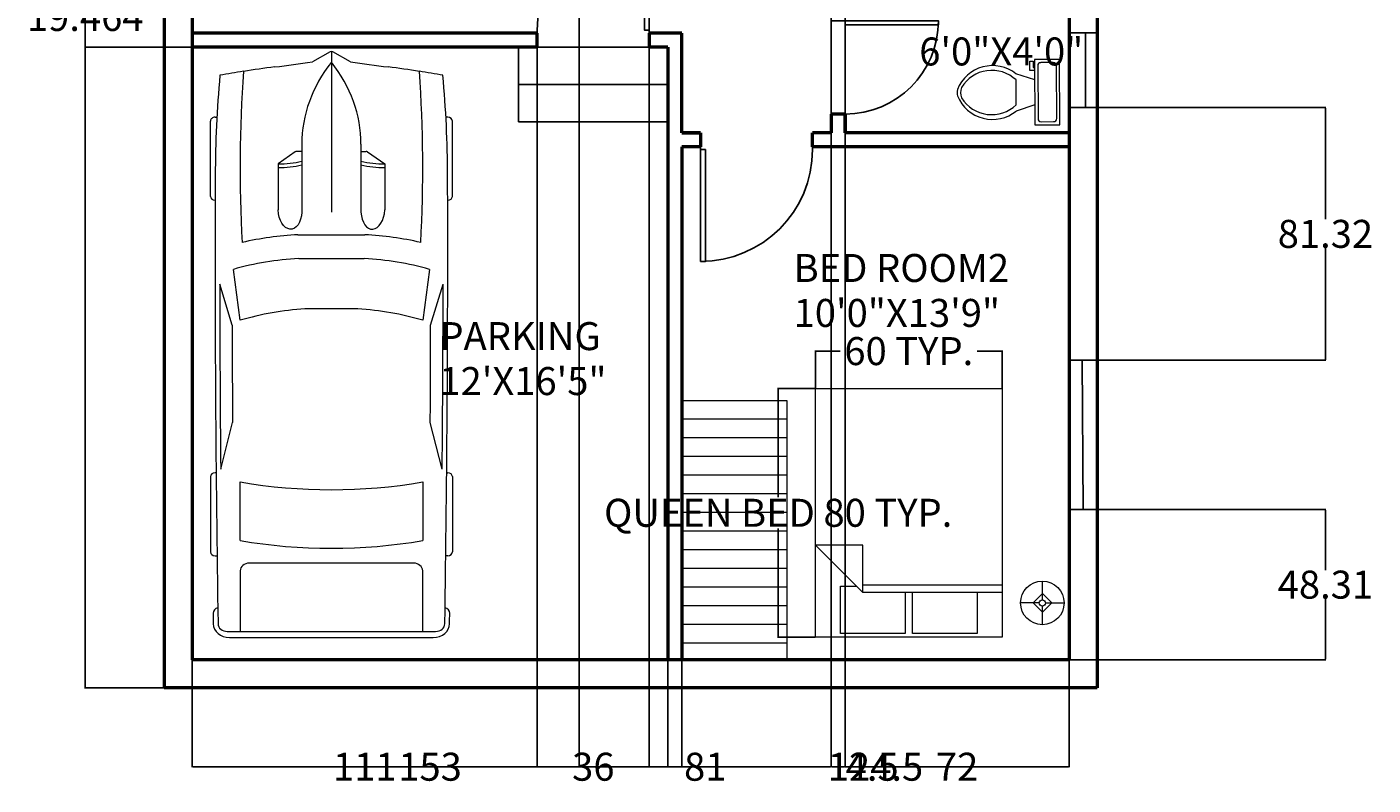
# Model space of a CAD drawing. Units: inches. Extents: x -49 to 419, y 83 to 650.
# Tile 1 of 2: x -14 to 419, y 83 to 327. Entities that reach past the tile are written whole.
import ezdxf

# ---------------------------------------------------------------- set-up
doc = ezdxf.new("R2010")
doc.units = ezdxf.units.IN
for name, color, linetype, lineweight in [('A-ANNO-DIMS', 2, 'Continuous', 18), ('A-AREA-IDEN', 2, 'Continuous', 25), ('A-DOOR', 20, 'Continuous', 25), ('A-FLOR-CASE', 130, 'Continuous', 18), ('A-FLOR-FIXT', 130, 'Continuous', 18), ('A-FLOR-STRS', 150, 'Continuous', 25), ('A-GLAZ', 70, 'Continuous', 25), ('A-SITE-VEHI', 130, 'Continuous', 13), ('FUR', 130, 'Continuous', 18), ('WAL', 210, 'Continuous', 50)]:
    doc.layers.add(name, color=color, linetype=linetype, lineweight=lineweight)
doc.styles.get("Standard").update_dxf_attribs({"font": 'arial.ttf', "height": 9})
doc.dimstyles.get("Standard").update_dxf_attribs({"dimtxt": 0.18, "dimasz": 0.18, "dimexe": 0.18, "dimexo": 0.0625, "dimgap": 0.09, "dimtad": 0, "dimtih": 1, "dimtoh": 1, "dimdec": 4, "dimzin": 0, "dimdsep": 46, "dimtxsty": 'Standard', "dimcen": 0.09, "dimadec": 0, "dimazin": 0, "dimtfac": 1, "dimtdec": 4, "dimtofl": 0, "dimtmove": 0, "dimatfit": 3, "dimfxl": 1, "dimtolj": 1, "dimtzin": 0, "dimarcsym": 0})

# ---------------------------------------------------------------- blocks, each defined once
blk = doc.blocks.new('*U2')
for p, q in [((0, 0), (0, -6)), ((40, 0), (40, -6))]:
    blk.add_line(p, q)
blk.add_lwpolyline([(0, 0), (0, 40), (1.75, 40), (1.75, 0)], close=True)
blk.add_arc((0, 0), 40, 0, 90)
blk = doc.blocks.new('*U4')
for p, q in [((9.5, -6), (9.5, -2)), ((-10, -8.5), (-8, -8.5)), ((-10, -9.5), (-10, -8.5)), ((-8, -8.5), (-8, -8)), ((-7, -8), (-7, -9.5)), ((-4, -8), (-6, -14)), ((4, -8), (6, -14)), ((-7, -9.5), (-10, -9.5)), ((4, -14), (-4, -14))]:
    blk.add_line(p, q)
blk.add_lwpolyline([(10.5, -8), (10.5, 0), (-10.5, 0), (-10.5, -8)], close=True)
for points in [[(-9.5, -2), (-9.5, -6)], [(8.5, -1), (-8.5, -1)], [(-8.5, -7), (8.5, -7)]]:
    blk.add_lwpolyline(points)
for centre, radius, start, end in [((-8.62, -1.88), 0.884, 81.8699, 188.1301), ((8.62, -1.88), 0.884, 351.8699, 98.1301), ((-8.62, -6.12), 0.884, 171.8699, 278.1301), ((8.62, -6.12), 0.884, 261.8699, 8.1301), ((3.52, -21.58), 12.17, 141.4691, 247.9714), ((4.2, -21.82), 11.33, 136.3677, 238.9468), ((-3.52, -21.58), 12.17, 292.0284, 38.5307), ((-4.2, -21.82), 11.33, 301.053, 43.6321), ((0, -27.88), 4, 245.7318, 294.2682), ((0, -29), 4, 254.8605, 285.1395)]:
    blk.add_arc(centre, radius, start, end)
blk = doc.blocks.new('Bed - Queen')
for p, q in [((0, -80.00003), (0, 0)), ((0, 0), (59.99999, 0)), ((59.99999, 0), (59.99999, -80.00003)), ((7.99999, -1.2), (28.79998, -1.2)), ((7.99999, -14.4), (7.99999, -1.2)), ((28.79998, -1.2), (28.79998, -14.4)), ((31.19999, -1.2), (51.99999, -1.2)), ((31.19999, -14.4), (31.19999, -1.2)), ((51.99999, -1.2), (51.99999, -16.4)), ((0, -14.4), (44.8, -14.4)), ((44.8, -16.8), (0, -16.8)), ((59.99999, -29.6), (44.8, -14.4)), ((44.8, -14.4), (44.8, -29.6)), ((51.99999, -16.4), (46.79936, -16.4)), ((44.8, -29.6), (59.99999, -29.6)), ((59.99999, -80.00003), (0, -80.00003))]:
    blk.add_line(p, q)
blk = doc.blocks.new('Lamp - Table')
for p, q in [((0, 7), (0, 1)), ((-1, 0), (-7, 0)), ((0, 3), (-3, 0)), ((-3, 0), (0, -3)), ((3, 0), (0, 3)), ((0, -3), (3, 0)), ((1, 0), (7, 0)), ((0, -1), (0, -7))]:
    blk.add_line(p, q)
for radius in [7, 1]:
    blk.add_circle((0, 0), radius)
blk = doc.blocks.new('*U11')
for p, q in [((21.1, 37.41), (21.1, 36.83)), ((46.55, 38.89), (22.35, 38.89)), ((47.8, 37.39), (47.8, 37.41)), ((87.99, 31.87), (74.76, 35.92)), ((134.31, 35.6), (119.29, 31.78)), ((135.45, 37.07), (135.45, 37.41)), ((136.7, 38.89), (160.9, 38.89)), ((162.15, 37.41), (162.15, 36.77)), ((70.03, 31.54), (86.41, 29.35)), ((186.47, -33.5), (186.47, 33.5)), ((188.4, -32.76), (188.4, 32.76)), ((138.42, 29.35), (157.25, 29.35)), ((164.52, 26.39), (164.52, -26.39)), ((186.47, 29.35), (167.01, 29.35)), ((32.27, 11.63), (36.13, 17.17)), ((36.13, 17.17), (50.94, 17.17)), ((29.77, 9.51), (51.68, 9.51)), ((32.12, 9.51), (32.12, 11.15)), ((58.92, -10.77), (58.92, 10.77)), ((66.55, -10.53), (66.55, 10.53)), ((186.47, -10.53), (186.47, 10.53)), ((3.27, 6.13), (0.1, 0.41)), ((82.74, 8.5), (82.74, -8.5)), ((0, 0), (51.68, 0)), ((0.1, -0.41), (3.27, -6.13)), ((29.77, -9.51), (51.68, -9.51)), ((32.12, -9.51), (32.12, -11.15)), ((32.27, -11.63), (36.13, -17.17)), ((36.13, -17.17), (50.94, -17.17)), ((86.41, -29.35), (70.03, -31.54)), ((157.25, -29.35), (138.42, -29.35)), ((167.01, -29.35), (186.47, -29.35)), ((87.99, -31.87), (74.76, -35.92)), ((134.31, -35.6), (119.29, -31.78)), ((21.1, -37.41), (21.1, -36.83)), ((46.55, -38.89), (22.35, -38.89)), ((47.8, -37.39), (47.8, -37.41)), ((135.45, -37.07), (135.45, -37.41)), ((136.7, -38.89), (160.9, -38.89)), ((162.15, -37.41), (162.15, -36.77))]:
    blk.add_line(p, q)
for centre, major_axis, ratio, start_param, end_param in [((266.03, -27.52), (0, 313.31), 0.842304, 1.367076, 1.39176), ((41.19, -490.86), (0, 528.23), 0.842304, 0.00281, 0.075598), ((22.35, 37.41), (0, -1.48), 0.842304, 3.141593, 4.712389), ((64.48, -10555.62), (0, 10593.03), 0.842304, -0.013397, 0.002797), ((46.55, 37.41), (0, 1.48), 0.842304, -1.570796, 0), ((64.48, -10555.62), (0, -10591.55), 0.842304, 3.133765, 3.140441), ((136.7, 37.41), (0, -1.48), 0.842304, 3.141593, 4.712389), ((160.9, 37.41), (0, 1.48), 0.842304, -1.570796, 0), ((180.63, 35.84), (0, 2.22), 0.842304, -0.013017, 1.249894), ((64.48, -10556.36), (0, 10595.31), 0.842304, -0.013397, -0.013017), ((183.98, 33.5), (0, -2.96), 0.842304, 1.570796, 3.128196), ((183.98, 32.76), (0, -5.25), 0.842304, 1.570796, 3.128196), ((135.29, 5.39), (0, 81.77), 0.842304, 1.245306, 1.50788), ((95.79, -3666.35), (0, -3698.24), 0.842304, 3.134049, 3.144098), ((259.18, -27.52), (0, -305.3), 0.842304, 4.528606, 4.561838), ((37.47, -593.96), (0, -623.33), 0.842304, 3.096046, 3.200911), ((134.4, 5.39), (0, -89.78), 0.842304, 4.449482, 4.652344), ((149.6, 2.8), (0, -79.58), 0.842304, 4.372215, 4.640744), ((17.08, 0), (0, 147.02), 0.842304, 4.511394, 4.913384), ((35.91, 0), (0, 147.02), 0.842304, 4.511394, 4.913384), ((167.01, 26.39), (0, 2.96), 0.842304, 0, 1.570796), ((-204.49, 52.4), (0, -250.96), 0.842304, 1.385369, 1.434372), ((13.04, 17.01), (0, 27.42), 0.842304, 4.435146, 4.718221), ((14.2, 17.01), (0, 27.42), 0.842304, 4.435146, 4.718221), ((50.79, 13.34), (6.34, -0.36), 0.603834, -1.395552, 1.581315), ((29.77, -46.66), (0, 56.17), 0.842304, 0, 0.590319), ((32.75, 11.15), (0, 0.74), 0.842304, 0.879714, 1.570796), ((0.62, 0), (0, -0.74), 0.842304, 4.131459, 5.293319), ((29.77, 46.66), (0, 56.17), 0.842304, 2.551274, 3.141593), ((-204.49, -52.4), (0, 250.96), 0.842304, -1.434372, -1.385369), ((149.6, -2.8), (0, -79.58), 0.842304, -1.499151, -1.230623), ((32.75, -11.15), (0, -0.74), 0.842304, 4.712389, 5.403472), ((13.04, -17.01), (0, -27.42), 0.842304, 1.564964, 1.848039), ((14.2, -17.01), (0, -27.42), 0.842304, 1.564964, 1.848039), ((134.4, -5.39), (0, -89.78), 0.842304, -1.510751, -1.307889), ((135.29, -5.39), (0, -81.77), 0.842304, -1.50788, -1.245306), ((259.18, 27.52), (0, 305.3), 0.842304, 1.721348, 1.754579), ((266.03, 27.52), (0, 313.31), 0.842304, 1.749832, 1.774517), ((37.47, 593.96), (0, -623.33), 0.842304, -0.059319, 0.045547), ((167.01, -26.39), (0, -2.96), 0.842304, 4.712389, 6.283185), ((95.79, 3666.35), (0, -3698.24), 0.842304, -0.002505, 0.007544), ((183.98, -33.5), (0, 2.96), 0.842304, 3.15499, 4.712389), ((183.98, -32.76), (0, -5.25), 0.842304, 0.013397, 1.570796), ((41.19, 490.86), (0, -528.23), 0.842304, -0.075598, -0.00281), ((22.35, -37.41), (0, 1.48), 0.842304, 1.570796, 3.141593), ((64.48, 10555.62), (0, 10593.03), 0.842304, 3.138796, 3.15499), ((46.55, -37.41), (0, -1.48), 0.842304, 0, 1.570796), ((64.48, 10555.62), (0, -10591.55), 0.842304, 0.001152, 0.007828), ((136.7, -37.41), (0, -1.48), 0.842304, -1.570796, 0), ((160.9, -37.41), (0, 1.48), 0.842304, 3.141593, 4.712389), ((180.63, -35.84), (0, -2.22), 0.842304, -1.249894, 0.013017), ((64.48, 10556.36), (0, 10595.31), 0.842304, 3.15461, 3.15499)]:
    blk.add_ellipse(centre, major_axis=major_axis, ratio=ratio, start_param=start_param, end_param=end_param)
at = {"extrusion": (0, 0, -1)}
blk.add_ellipse((50.79, -13.34), major_axis=(6.34, 0.36), ratio=0.603834, start_param=-1.395552, end_param=1.581315, dxfattribs=at)
blk = doc.blocks.new('WIN-48IN')
for p, q in [((0, 48), (0, 0)), ((9, 48), (0, 48)), ((4.19, 48), (4.5, 0)), ((9, 0), (9, 48)), ((0, 0), (9, 0))]:
    blk.add_line(p, q)
blk = doc.blocks.new('WIN-24IN')
for p, q in [((0, 24), (0, 0)), ((9, 24), (0, 24)), ((0, 24), (5.33, 24)), ((5.33, 24), (5.33, 0)), ((9, 0), (9, 24)), ((0, 0), (9, 0))]:
    blk.add_line(p, q)
blk = doc.blocks.new('*D18')
at = {"layer": 'A-ANNO-DIMS', "color": 0, "lineweight": -2, "transparency": 16777216}
for p, q in [((239.4, 210.27), (227.28, 210.27)), ((227.46, 210.09), (227.46, 175.29)), ((227.46, 130.45), (227.46, 165.25)), ((239.4, 130.27), (227.28, 130.27))]:
    blk.add_line(p, q, dxfattribs=at)
at = {"layer": 'A-ANNO-DIMS', "color": 0, "transparency": 16777216}
for points in [[(227.43, 210.09), (227.49, 210.09), (227.46, 210.27)], [(227.43, 130.45), (227.49, 130.45), (227.46, 130.27)]]:
    blk.add_solid(points, dxfattribs=at)
at = {"layer": 'Defpoints', "color": 0, "transparency": 16777216}
for p in [(239.46, 210.27), (227.46, 130.27), (239.46, 130.27)]:
    blk.add_point(p, dxfattribs=at)
at = {"layer": 'A-ANNO-DIMS', "color": 0, "transparency": 16777216, "insert": (227.46, 170.27), "char_height": 9, "attachment_point": 5}
blk.add_mtext('\\A1;QUEEN BED 80 TYP.', dxfattribs=at)
blk = doc.blocks.new('*D19')
at = {"layer": 'A-ANNO-DIMS', "color": 0, "lineweight": -2, "transparency": 16777216}
for p, q in [((239.46, 210.33), (239.46, 222.45)), ((239.64, 222.27), (247.44, 222.27)), ((299.28, 222.27), (291.48, 222.27)), ((299.46, 210.33), (299.46, 222.45))]:
    blk.add_line(p, q, dxfattribs=at)
at = {"layer": 'A-ANNO-DIMS', "color": 0, "transparency": 16777216}
for points in [[(239.64, 222.3), (239.64, 222.24), (239.46, 222.27)], [(299.28, 222.3), (299.28, 222.24), (299.46, 222.27)]]:
    blk.add_solid(points, dxfattribs=at)
at = {"layer": 'Defpoints', "color": 0, "transparency": 16777216}
for p in [(239.46, 222.27), (239.46, 210.27), (299.46, 210.27)]:
    blk.add_point(p, dxfattribs=at)
at = {"layer": 'A-ANNO-DIMS', "color": 0, "transparency": 16777216, "insert": (269.46, 222.27), "char_height": 9, "attachment_point": 5}
blk.add_mtext('\\A1;60 TYP.', dxfattribs=at)
blk = doc.blocks.new('*D27')
at = {"layer": 'A-ANNO-DIMS', "color": 0, "lineweight": -2, "transparency": 16777216}
for p, q in [((29.94, 570), (4.42, 570)), ((4.6, 569.82), (4.6, 346.69)), ((4.6, 114.18), (4.6, 337.31)), ((29.94, 114), (4.42, 114))]:
    blk.add_line(p, q, dxfattribs=at)
at = {"layer": 'A-ANNO-DIMS', "color": 0, "transparency": 16777216}
for points in [[(4.57, 569.82), (4.63, 569.82), (4.6, 570)], [(4.57, 114.18), (4.63, 114.18), (4.6, 114)]]:
    blk.add_solid(points, dxfattribs=at)
at = {"layer": 'Defpoints', "color": 0, "transparency": 16777216}
for p in [(4.6, 570), (30, 570), (30, 114)]:
    blk.add_point(p, dxfattribs=at)
at = {"layer": 'A-ANNO-DIMS', "color": 0, "transparency": 16777216, "insert": (4.6, 342), "char_height": 9, "attachment_point": 5}
blk.add_mtext('\\A1;456', dxfattribs=at)
blk = doc.blocks.new('*D28')
at = {"layer": 'A-ANNO-DIMS', "color": 0, "lineweight": -2, "transparency": 16777216}
for p, q in [((321.06, 171.31), (403.62, 171.31)), ((403.44, 171.13), (403.44, 151.84)), ((403.44, 123.18), (403.44, 142.47)), ((321.06, 123), (403.62, 123))]:
    blk.add_line(p, q, dxfattribs=at)
at = {"layer": 'A-ANNO-DIMS', "color": 0, "transparency": 16777216}
for points in [[(403.41, 171.13), (403.47, 171.13), (403.44, 171.31)], [(403.41, 123.18), (403.47, 123.18), (403.44, 123)]]:
    blk.add_solid(points, dxfattribs=at)
at = {"layer": 'Defpoints', "color": 0, "transparency": 16777216}
for p in [(321, 171.31), (403.44, 171.31), (321, 123)]:
    blk.add_point(p, dxfattribs=at)
at = {"layer": 'A-ANNO-DIMS', "color": 0, "transparency": 16777216, "insert": (403.44, 147.16), "char_height": 9, "attachment_point": 5}
blk.add_mtext('\\A1;48.31', dxfattribs=at)
blk = doc.blocks.new('*D29')
at = {"layer": 'A-ANNO-DIMS', "color": 0, "lineweight": -2, "transparency": 16777216}
for p, q in [((321.06, 300.63), (403.62, 300.63)), ((403.44, 300.45), (403.44, 264.66)), ((403.44, 219.49), (403.44, 255.28)), ((321.06, 219.31), (403.62, 219.31))]:
    blk.add_line(p, q, dxfattribs=at)
at = {"layer": 'A-ANNO-DIMS', "color": 0, "transparency": 16777216}
for points in [[(403.41, 300.45), (403.47, 300.45), (403.44, 300.63)], [(403.41, 219.49), (403.47, 219.49), (403.44, 219.31)]]:
    blk.add_solid(points, dxfattribs=at)
at = {"layer": 'Defpoints', "color": 0, "transparency": 16777216}
for p in [(321, 300.63), (403.44, 300.63), (321, 219.31)]:
    blk.add_point(p, dxfattribs=at)
at = {"layer": 'A-ANNO-DIMS', "color": 0, "transparency": 16777216, "insert": (403.44, 259.97), "char_height": 9, "attachment_point": 5}
blk.add_mtext('\\A1;81.32', dxfattribs=at)
blk = doc.blocks.new('*D30')
at = {"layer": 'A-ANNO-DIMS', "color": 0, "lineweight": -2, "transparency": 16777216}
for p, q in [((29.94, 339.46), (4.42, 339.46)), ((4.6, 339.28), (4.6, 334.42)), ((4.6, 320.18), (4.6, 325.05)), ((38.94, 320), (4.42, 320))]:
    blk.add_line(p, q, dxfattribs=at)
at = {"layer": 'A-ANNO-DIMS', "color": 0, "transparency": 16777216}
for points in [[(4.57, 339.28), (4.63, 339.28), (4.6, 339.46)], [(4.57, 320.18), (4.63, 320.18), (4.6, 320)]]:
    blk.add_solid(points, dxfattribs=at)
at = {"layer": 'Defpoints', "color": 0, "transparency": 16777216}
for p in [(30, 339.46), (4.6, 320), (39, 320)]:
    blk.add_point(p, dxfattribs=at)
at = {"layer": 'A-ANNO-DIMS', "color": 0, "transparency": 16777216, "insert": (4.6, 329.73), "char_height": 9, "attachment_point": 5}
blk.add_mtext('\\A1;19.464', dxfattribs=at)
blk = doc.blocks.new('*D34')
at = {"layer": 'A-ANNO-DIMS', "color": 0, "lineweight": -2, "transparency": 16777216}
for p, q in [((39, 122.94), (39, 88.42)), ((192, 122.94), (192, 88.42)), ((39.18, 88.6), (105.89, 88.6)), ((191.82, 88.6), (125.11, 88.6))]:
    blk.add_line(p, q, dxfattribs=at)
at = {"layer": 'A-ANNO-DIMS', "color": 0, "transparency": 16777216}
for points in [[(39.18, 88.63), (39.18, 88.57), (39, 88.6)], [(191.82, 88.63), (191.82, 88.57), (192, 88.6)]]:
    blk.add_solid(points, dxfattribs=at)
at = {"layer": 'Defpoints', "color": 0, "transparency": 16777216}
for p in [(39, 123), (192, 123), (192, 88.6)]:
    blk.add_point(p, dxfattribs=at)
at = {"layer": 'A-ANNO-DIMS', "color": 0, "transparency": 16777216, "insert": (115.5, 88.6), "char_height": 9, "attachment_point": 5}
blk.add_mtext('\\A1;153', dxfattribs=at)
blk = doc.blocks.new('*D35')
at = {"layer": 'A-ANNO-DIMS', "color": 0, "lineweight": -2, "transparency": 16777216}
for p, q in [((196.5, 122.94), (196.5, 88.42)), ((321, 122.94), (321, 88.42)), ((196.68, 88.6), (243.86, 88.6)), ((320.82, 88.6), (273.64, 88.6))]:
    blk.add_line(p, q, dxfattribs=at)
at = {"layer": 'A-ANNO-DIMS', "color": 0, "transparency": 16777216}
for points in [[(196.68, 88.63), (196.68, 88.57), (196.5, 88.6)], [(320.82, 88.63), (320.82, 88.57), (321, 88.6)]]:
    blk.add_solid(points, dxfattribs=at)
at = {"layer": 'Defpoints', "color": 0, "transparency": 16777216}
for p in [(196.5, 123), (321, 123), (321, 88.6)]:
    blk.add_point(p, dxfattribs=at)
at = {"layer": 'A-ANNO-DIMS', "color": 0, "transparency": 16777216, "insert": (258.75, 88.6), "char_height": 9, "attachment_point": 5}
blk.add_mtext('\\A1;124.5', dxfattribs=at)
blk = doc.blocks.new('*D36')
at = {"layer": 'A-ANNO-DIMS', "color": 0, "lineweight": -2, "transparency": 16777216}
for p, q in [((163.5, 500.94), (163.5, 88.42)), ((244.5, 500.94), (244.5, 88.42)), ((163.68, 88.6), (198.33, 88.6)), ((244.32, 88.6), (209.67, 88.6))]:
    blk.add_line(p, q, dxfattribs=at)
at = {"layer": 'A-ANNO-DIMS', "color": 0, "transparency": 16777216}
for points in [[(163.68, 88.63), (163.68, 88.57), (163.5, 88.6)], [(244.32, 88.63), (244.32, 88.57), (244.5, 88.6)]]:
    blk.add_solid(points, dxfattribs=at)
at = {"layer": 'Defpoints', "color": 0, "transparency": 16777216}
for p in [(163.5, 501), (244.5, 501), (244.5, 88.6)]:
    blk.add_point(p, dxfattribs=at)
at = {"layer": 'A-ANNO-DIMS', "color": 0, "transparency": 16777216, "insert": (204, 88.6), "char_height": 9, "attachment_point": 5}
blk.add_mtext('\\A1;81', dxfattribs=at)
blk = doc.blocks.new('*D37')
at = {"layer": 'A-ANNO-DIMS', "color": 0, "lineweight": -2, "transparency": 16777216}
for p, q in [((249, 440.94), (249, 88.42)), ((321, 440.94), (321, 88.42)), ((249.18, 88.6), (278.55, 88.6)), ((320.82, 88.6), (291.45, 88.6))]:
    blk.add_line(p, q, dxfattribs=at)
at = {"layer": 'A-ANNO-DIMS', "color": 0, "transparency": 16777216}
for points in [[(249.18, 88.63), (249.18, 88.57), (249, 88.6)], [(320.82, 88.63), (320.82, 88.57), (321, 88.6)]]:
    blk.add_solid(points, dxfattribs=at)
at = {"layer": 'Defpoints', "color": 0, "transparency": 16777216}
for p in [(249, 441), (321, 441), (321, 88.6)]:
    blk.add_point(p, dxfattribs=at)
at = {"layer": 'A-ANNO-DIMS', "color": 0, "transparency": 16777216, "insert": (285, 88.6), "char_height": 9, "attachment_point": 5}
blk.add_mtext('\\A1;72', dxfattribs=at)
blk = doc.blocks.new('*D44')
at = {"layer": 'A-ANNO-DIMS', "color": 0, "lineweight": -2, "transparency": 16777216}
for p, q in [((244.5, 482.94), (244.5, 88.42)), ((249, 482.94), (249, 88.42)), ((244.68, 88.6), (248.82, 88.6)), ((249, 88.6), (249.18, 88.6))]:
    blk.add_line(p, q, dxfattribs=at)
at = {"layer": 'A-ANNO-DIMS', "color": 0, "transparency": 16777216}
for points in [[(244.68, 88.63), (244.68, 88.57), (244.5, 88.6)], [(248.82, 88.63), (248.82, 88.57), (249, 88.6)]]:
    blk.add_solid(points, dxfattribs=at)
at = {"layer": 'Defpoints', "color": 0, "transparency": 16777216}
for p in [(244.5, 483), (249, 483), (249, 88.6)]:
    blk.add_point(p, dxfattribs=at)
at = {"layer": 'A-ANNO-DIMS', "color": 0, "transparency": 16777216, "insert": (257.68, 88.6), "char_height": 9, "attachment_point": 5}
blk.add_mtext('\\A1;4.5', dxfattribs=at)
blk = doc.blocks.new('*D45')
at = {"layer": 'A-ANNO-DIMS', "color": 0, "lineweight": -2, "transparency": 16777216}
for p, q in [((150, 319.94), (150, 88.42)), ((186, 319.94), (186, 88.42)), ((150.18, 88.6), (161.47, 88.6)), ((185.82, 88.6), (174.53, 88.6))]:
    blk.add_line(p, q, dxfattribs=at)
at = {"layer": 'A-ANNO-DIMS', "color": 0, "transparency": 16777216}
for points in [[(150.18, 88.63), (150.18, 88.57), (150, 88.6)], [(185.82, 88.63), (185.82, 88.57), (186, 88.6)]]:
    blk.add_solid(points, dxfattribs=at)
at = {"layer": 'Defpoints', "color": 0, "transparency": 16777216}
for p in [(150, 320), (186, 320), (186, 88.6)]:
    blk.add_point(p, dxfattribs=at)
at = {"layer": 'A-ANNO-DIMS', "color": 0, "transparency": 16777216, "insert": (168, 88.6), "char_height": 9, "attachment_point": 5}
blk.add_mtext('\\A1;36', dxfattribs=at)
blk = doc.blocks.new('*D46')
at = {"layer": 'A-ANNO-DIMS', "color": 0, "lineweight": -2, "transparency": 16777216}
for p, q in [((39, 319.94), (39, 88.42)), ((150, 319.94), (150, 88.42)), ((39.18, 88.6), (85.76, 88.6)), ((149.82, 88.6), (103.24, 88.6))]:
    blk.add_line(p, q, dxfattribs=at)
at = {"layer": 'A-ANNO-DIMS', "color": 0, "transparency": 16777216}
for points in [[(39.18, 88.63), (39.18, 88.57), (39, 88.6)], [(149.82, 88.63), (149.82, 88.57), (150, 88.6)]]:
    blk.add_solid(points, dxfattribs=at)
at = {"layer": 'Defpoints', "color": 0, "transparency": 16777216}
for p in [(39, 320), (150, 320), (150, 88.6)]:
    blk.add_point(p, dxfattribs=at)
at = {"layer": 'A-ANNO-DIMS', "color": 0, "transparency": 16777216, "insert": (94.5, 88.6), "char_height": 9, "attachment_point": 5}
blk.add_mtext('\\A1;111', dxfattribs=at)

msp = doc.modelspace()

# ---------------------------------------------------------------- linework, layer by layer
at = {"layer": 'A-FLOR-CASE'}
for p, q in [((230.3491, 206.3248), (196.5, 206.3248)), ((230.3491, 123), (230.3491, 206.3248)), ((230.3491, 200.3248), (196.5, 200.3248)), ((230.3491, 194.3248), (196.5, 194.3248)), ((230.3491, 188.3248), (196.5, 188.3248)), ((230.3491, 182.3248), (196.5, 182.3248)), ((230.3491, 176.3248), (196.5, 176.3248)), ((230.3491, 170.3248), (196.5, 170.3248)), ((230.3491, 164.3248), (196.5, 164.3248)), ((230.3491, 158.3248), (196.5, 158.3248)), ((230.3491, 152.3248), (196.5, 152.3248)), ((230.3491, 146.3248), (196.5, 146.3248)), ((230.3491, 140.3248), (196.5, 140.3248)), ((230.3491, 134.3248), (196.5, 134.3248)), ((230.3491, 128.3248), (196.5, 128.3248))]:
    msp.add_line(p, q, dxfattribs=at)
at = {"layer": 'A-FLOR-STRS'}
for p, q in [((186, 320), (143.9905, 320)), ((143.9905, 320), (143.9905, 296)), ((192, 308), (143.9905, 308)), ((192, 296), (192, 308)), ((143.9905, 296), (192, 296))]:
    msp.add_line(p, q, dxfattribs=at)
at = {"layer": 'WAL'}
for p, q in [((30, 570), (30, 114)), ((330, 570), (330, 114)), ((39, 561), (39, 123)), ((321, 561), (321, 123)), ((150, 324.5), (39, 324.5)), ((150, 320), (150, 324.5)), ((192, 324.5), (186, 324.5)), ((192, 324.5), (186, 324.5)), ((186, 324.5), (186, 320)), ((196.5, 324.5302), (192, 324.5302)), ((196.5, 292.5), (196.5, 324.5302)), ((150, 320), (39, 320)), ((192, 320), (186, 320)), ((192, 320), (192, 123)), ((249, 298.5), (244.5, 298.5)), ((244.5, 298.5), (244.5, 292.5)), ((249, 292.5), (249, 298.5)), ((249, 298.5), (249, 292.5)), ((196.5, 292.5), (202.5, 292.5)), ((202.5, 292.5), (196.5, 292.5)), ((202.5, 292.5), (202.5, 288)), ((238.5, 288), (238.5, 292.5)), ((244.5, 292.5), (238.5, 292.5)), ((321, 292.5), (249, 292.5)), ((196.5, 288), (196.5, 123)), ((202.5, 288), (196.5, 288)), ((321, 288), (238.5, 288)), ((321, 123), (39, 123)), ((330, 114), (30, 114))]:
    msp.add_line(p, q, dxfattribs=at)

# ---------------------------------------------------------------- block references
at = {"layer": 'A-DOOR', "xscale": -0.9, "yscale": 0.9, "zscale": 0.9}
msp.add_blockref('*U2', (186, 325.5224), dxfattribs=at)
at = {"layer": 'A-DOOR'}
for p, xscale, yscale, zscale, rotation in [((249, 328.5), 0.75, 0.75, 0.75, 270), ((202.5, 287.1), -0.9, 0.9, 0.9, 180)]:
    msp.add_blockref('*U2', p, dxfattribs=dict(at, xscale=xscale, yscale=yscale, zscale=zscale, rotation=rotation))
at = {"layer": 'A-FLOR-FIXT', "rotation": 270.3584011672319}
msp.add_blockref('*U4', (317.9711, 305.5748), dxfattribs=at)
at = {"layer": 'A-GLAZ'}
for name, p in [('WIN-24IN', (321, 300.629)), ('WIN-48IN', (321, 171.3105))]:
    msp.add_blockref(name, p, dxfattribs=at)
at = {"layer": 'A-SITE-VEHI', "rotation": 270}
msp.add_blockref('*U11', (83.7818, 318.593), dxfattribs=at)
at = {"layer": 'FUR', "rotation": 180}
for name, p in [('Bed - Queen', (299.4596, 130.2654)), ('Lamp - Table', (312.4086, 141.2788))]:
    msp.add_blockref(name, p, dxfattribs=at)

# ---------------------------------------------------------------- texts
at = {"layer": 'A-AREA-IDEN'}
for s, p in [('6\'0"X4\'0"', (272.822, 314.1326)), ('BED ROOM2', (232.4228, 244.5019)), ('10\'0"X13\'9"', (232.4228, 230.0442)), ('PARKING ', (118.5001, 222.5858)), ('12\'X16\'5"', (118.5001, 208.1281))]:
    msp.add_text(s, height=9, dxfattribs=at).set_placement(p)

# ---------------------------------------------------------------- dimensions: what is measured, and where the dimension line sits
at = {"layer": 'A-ANNO-DIMS'}
for base, p1, p2, override, picture, middle in [((4.6, 570), (30, 114), (30, 570), {"dimdec": 0, "dimlfac": 1, "dimrnd": 0, "dimzin": 0, "dimdsep": 46, "dimlunit": 2}, '*D27', (4.6, 342)), ((4.6, 320), (30, 339.4638), (39, 320), {"dimdec": 3, "dimlfac": 1, "dimrnd": 0, "dimzin": 0, "dimdsep": 46, "dimlunit": 2}, '*D30', (4.6, 329.7319)), ((403.4356, 300.6286), (321, 219.3103), (321, 300.6286), {"dimdec": 2, "dimlfac": 1, "dimrnd": 0, "dimzin": 0, "dimdsep": 46, "dimlunit": 2}, '*D29', (403.4356, 259.9695)), ((403.4356, 171.3103), (321, 123), (321, 171.3103), {"dimdec": 2, "dimlfac": 1, "dimrnd": 0, "dimzin": 0, "dimdsep": 46, "dimlunit": 2}, '*D28', (403.4356, 147.1551))]:
    dim = msp.add_linear_dim(base=base, p1=p1, p2=p2, angle=90, dimstyle='Standard', override=override, dxfattribs=at)
    dim.commit()
    dim.dimension.update_dxf_attribs({"geometry": picture, "text_midpoint": middle})
for base, p1, p2, override, picture, middle in [((244.5, 88.6), (163.5, 501), (244.5, 501), {"dimdec": 0, "dimlfac": 1, "dimrnd": 0, "dimzin": 0, "dimdsep": 46, "dimlunit": 2}, '*D36', (204, 88.6)), ((249, 88.6), (244.5, 483), (249, 483), {"dimdec": 1, "dimlfac": 1, "dimrnd": 0, "dimzin": 0, "dimdsep": 46, "dimlunit": 2}, '*D44', (257.6776, 88.6)), ((321, 88.6), (249, 441), (321, 441), {"dimdec": 0, "dimlfac": 1, "dimrnd": 0, "dimzin": 0, "dimdsep": 46, "dimlunit": 2}, '*D37', (285, 88.6)), ((150, 88.6), (39, 320), (150, 320), {"dimdec": 0, "dimlfac": 1, "dimrnd": 0, "dimzin": 0, "dimdsep": 46, "dimlunit": 2}, '*D46', (94.5, 88.6)), ((186, 88.6), (150, 320), (186, 320), {"dimdec": 0, "dimlfac": 1, "dimrnd": 0, "dimzin": 0, "dimdsep": 46, "dimlunit": 2}, '*D45', (168, 88.6)), ((192, 88.6), (39, 123), (192, 123), {"dimdec": 0, "dimlfac": 1, "dimrnd": 0, "dimzin": 0, "dimdsep": 46, "dimlunit": 2}, '*D34', (115.5, 88.6)), ((321, 88.6), (196.5, 123), (321, 123), {"dimdec": 1, "dimlfac": 1, "dimrnd": 0, "dimzin": 0, "dimdsep": 46, "dimlunit": 2}, '*D35', (258.75, 88.6))]:
    dim = msp.add_linear_dim(base=base, p1=p1, p2=p2, dimstyle='Standard', override=override, dxfattribs=at)
    dim.commit()
    dim.dimension.update_dxf_attribs({"geometry": picture, "text_midpoint": middle})
for base, p1, p2, angle, text, picture, middle in [((239.4596, 222.2655), (299.4596, 210.2655), (239.4596, 210.2655), 180, '<> TYP.', '*D19', (269.4596, 222.2655)), ((227.4596, 130.2654), (239.4596, 210.2655), (239.4596, 130.2654), 270, 'QUEEN BED <> TYP.', '*D18', (227.4596, 170.2654))]:
    dim = msp.add_linear_dim(base=base, p1=p1, p2=p2, angle=angle, text=text, dimstyle='Standard', override={"dimdec": 0, "dimlfac": 1, "dimrnd": 0, "dimzin": 0, "dimdsep": 46, "dimlunit": 2}, dxfattribs=at)
    dim.commit()
    dim.dimension.update_dxf_attribs({"geometry": picture, "text_midpoint": middle})

doc.saveas('drawing.dxf')
